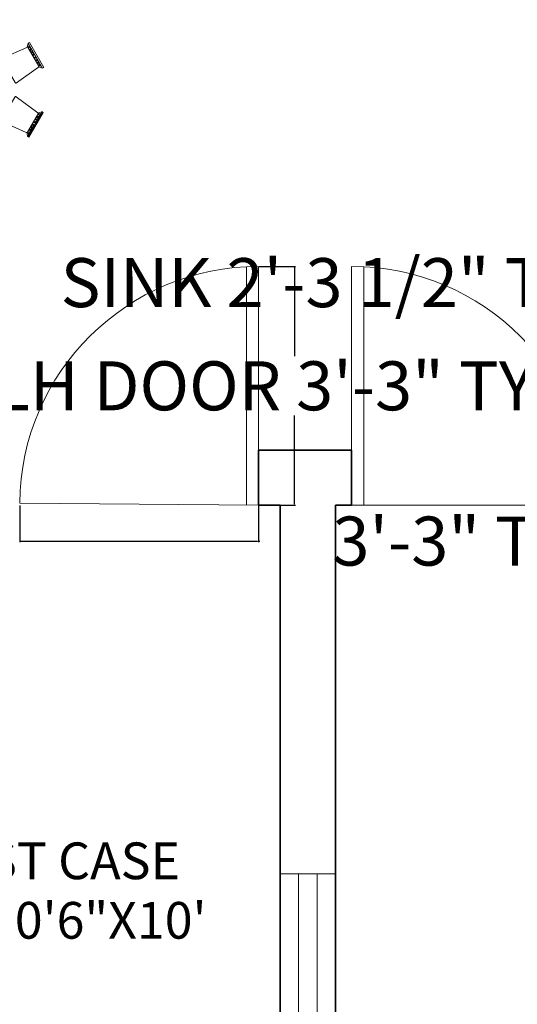
# Model space of a CAD drawing. Units: inches. Extents: x 125 to 976, y 231 to 853.
# Tile 14 of 16: x 655 to 736, y 413 to 573. Entities that reach past the tile are written whole.
import ezdxf

# ---------------------------------------------------------------- set-up
doc = ezdxf.new("R2010")
doc.units = ezdxf.units.IN
doc.header["$MEASUREMENT"] = 0
for name, color, linetype, lineweight in [('A-ANNO-DIMS', 2, 'Continuous', 18), ('A-AREA-IDEN', 7, 'Continuous', 18), ('A-DOOR', 3, 'Continuous', 18), ('A-GLAZ', 4, 'Continuous', 18), ('A-WALL', 7, 'Continuous', 35), ('Furniture', 8, 'Continuous', 15)]:
    doc.layers.add(name, color=color, linetype=linetype, lineweight=lineweight)
doc.styles.get("Standard").update_dxf_attribs({"font": 'italic8.shx'})
doc.dimstyles.get("Standard").update_dxf_attribs({"dimtxt": 8, "dimasz": 0.18, "dimexe": 0.18, "dimexo": 0.0625, "dimgap": 0.09, "dimtad": 0, "dimtih": 1, "dimtoh": 1, "dimdec": 4, "dimzin": 0, "dimdsep": 46, "dimlunit": 3, "dimtxsty": 'Standard', "dimcen": 0.09, "dimclrt": 4, "dimadec": 0, "dimazin": 0, "dimtfac": 1, "dimtdec": 4, "dimtofl": 0, "dimtmove": 0, "dimatfit": 3, "dimfxl": 1, "dimtolj": 1, "dimtzin": 0, "dimarcsym": 0})

# ---------------------------------------------------------------- blocks, each defined once
blk = doc.blocks.new('DINING-SET-ROUND-6')
for p, q in [((8.8, 22.58), (9.2, 22.26)), ((8.83, 22.8), (8.83, 22.6)), ((13.52, 22.8), (8.83, 22.8)), ((8.83, 22.6), (13.52, 22.6)), ((9.19, 22.53), (9.57, 22.55)), ((9.54, 22.27), (9.19, 22.53)), ((9.57, 22.55), (9.56, 22.32)), ((9.67, 22.56), (9.91, 22.32)), ((9.8, 22.55), (9.89, 22.55)), ((10.04, 22.32), (9.8, 22.55)), ((9.89, 22.55), (10.01, 22.45)), ((10.15, 22.56), (10.39, 22.32)), ((10.28, 22.55), (10.37, 22.55)), ((10.52, 22.32), (10.28, 22.55)), ((10.37, 22.55), (10.49, 22.45)), ((10.63, 22.56), (10.87, 22.32)), ((10.76, 22.55), (10.86, 22.55)), ((11, 22.32), (10.76, 22.55)), ((10.86, 22.55), (10.97, 22.45)), ((11.32, 22.32), (11.56, 22.55)), ((11.47, 22.55), (11.35, 22.45)), ((11.69, 22.56), (11.45, 22.32)), ((11.56, 22.55), (11.47, 22.55)), ((11.8, 22.32), (12.04, 22.55)), ((11.95, 22.55), (11.83, 22.45)), ((12.17, 22.56), (11.93, 22.32)), ((12.04, 22.55), (11.95, 22.55)), ((12.28, 22.32), (12.52, 22.55)), ((12.43, 22.55), (12.32, 22.45)), ((12.65, 22.56), (12.41, 22.32)), ((12.52, 22.55), (12.43, 22.55)), ((12.75, 22.55), (12.77, 22.32)), ((13.13, 22.53), (12.75, 22.55)), ((12.78, 22.27), (13.13, 22.53)), ((13.52, 22.58), (13.12, 22.26)), ((13.52, 22.6), (13.52, 22.8)), ((8.82, 17.72), (9.3, 22.08)), ((9.2, 22.26), (9.54, 22.27)), ((9.46, 22.23), (12.91, 22.23)), ((9.91, 22.32), (10.04, 22.32)), ((10.01, 22.45), (10.04, 22.48)), ((10.04, 22.48), (10.05, 22.34)), ((10.39, 22.32), (10.52, 22.32)), ((10.49, 22.45), (10.52, 22.48)), ((10.52, 22.48), (10.54, 22.34)), ((10.87, 22.32), (11, 22.32)), ((10.97, 22.45), (11, 22.48)), ((11, 22.48), (11.02, 22.34)), ((11.32, 22.48), (11.31, 22.34)), ((11.35, 22.45), (11.32, 22.48)), ((11.45, 22.32), (11.32, 22.32)), ((11.8, 22.48), (11.79, 22.34)), ((11.83, 22.45), (11.8, 22.48)), ((11.93, 22.32), (11.8, 22.32)), ((12.28, 22.48), (12.27, 22.34)), ((12.32, 22.45), (12.28, 22.48)), ((12.41, 22.32), (12.28, 22.32)), ((13.12, 22.26), (12.78, 22.27)), ((13.07, 22.08), (13.49, 17.72)), ((2.44, 19.22), (0.09, 15.16)), ((0.27, 15.05), (2.62, 19.11)), ((0.91, 15.41), (2.63, 18.4)), ((1.92, 17.81), (1.87, 17.73)), ((1.87, 17.73), (1.9, 17.58)), ((1.99, 17.49), (1.92, 17.81)), ((1.97, 17.93), (2.06, 17.6)), ((2.14, 18), (2.1, 17.99)), ((2.1, 17.99), (2.21, 17.9)), ((2.16, 18.23), (2.11, 18.14)), ((2.11, 18.14), (2.14, 18)), ((2.24, 17.91), (2.16, 18.23)), ((2.21, 18.35), (2.3, 18.02)), ((2.3, 18.02), (2.24, 17.91)), ((2.48, 18.75), (2.27, 18.42)), ((2.27, 18.42), (2.48, 18.32)), ((2.62, 19.11), (2.44, 19.22)), ((2.53, 18.31), (2.48, 18.75)), ((2.71, 18.6), (2.53, 18.31)), ((2.63, 19.1), (2.71, 18.6)), ((2.84, 18.46), (6.82, 16.65)), ((15.42, 16.53), (19.43, 18.29)), ((19.62, 18.97), (19.54, 18.47)), ((19.54, 18.47), (19.72, 18.18)), ((19.64, 18.23), (21.36, 15.24)), ((19.83, 19.06), (19.65, 18.95)), ((19.65, 18.95), (21.99, 14.9)), ((19.72, 18.18), (19.77, 18.62)), ((19.77, 18.62), (19.97, 18.29)), ((19.97, 18.29), (19.77, 18.19)), ((22.17, 15), (19.83, 19.06)), ((20.03, 18.21), (19.95, 17.89)), ((19.95, 17.89), (20.01, 17.77)), ((20.01, 17.77), (20.08, 18.1)), ((20.15, 17.86), (20.03, 17.77)), ((20.08, 18.1), (20.13, 18.01)), ((20.13, 18.01), (20.11, 17.87)), ((20.11, 17.87), (20.15, 17.86)), ((20.28, 17.8), (20.19, 17.47)), ((0.96, 16.18), (1.29, 16.27)), ((1.35, 16.38), (1.04, 16.28)), ((1.04, 16.28), (1.09, 16.36)), ((1.09, 16.36), (1.23, 16.41)), ((1.2, 16.59), (1.53, 16.68)), ((1.23, 16.41), (1.21, 16.46)), ((1.21, 16.46), (1.35, 16.4)), ((1.59, 16.79), (1.28, 16.7)), ((1.28, 16.7), (1.33, 16.78)), ((1.29, 16.27), (1.35, 16.38)), ((1.33, 16.78), (1.47, 16.83)), ((1.45, 16.87), (1.59, 16.82)), ((1.47, 16.83), (1.45, 16.87)), ((1.53, 16.68), (1.59, 16.79)), ((1.66, 17.16), (1.62, 17.15)), ((1.62, 17.15), (1.73, 17.07)), ((1.68, 17.39), (1.63, 17.31)), ((1.63, 17.31), (1.66, 17.16)), ((1.75, 17.07), (1.68, 17.39)), ((1.73, 17.51), (1.82, 17.18)), ((1.82, 17.18), (1.75, 17.07)), ((1.9, 17.58), (1.86, 17.57)), ((1.86, 17.57), (1.97, 17.48)), ((2.06, 17.6), (1.99, 17.49)), ((6.9, 16.42), (4.72, 12.66)), ((13.33, 17.54), (8.98, 17.54)), ((10.97, 16.52, 0.91), (10.97, 14.61, 0.91)), ((11.03, 16.52, 0.91), (10.97, 16.52, 0.91)), ((11.03, 14.61, 0.91), (11.03, 16.52, 0.91)), ((11.08, 16.52, 0.91), (11.08, 14.61, 0.91)), ((11.14, 16.52, 0.91), (11.08, 16.52, 0.91)), ((11.14, 14.61, 0.91), (11.14, 16.52, 0.91)), ((17.52, 12.54), (15.34, 16.3)), ((20.19, 17.47), (20.25, 17.36)), ((20.25, 17.36), (20.33, 17.68)), ((20.39, 17.44), (20.27, 17.35)), ((20.33, 17.68), (20.37, 17.6)), ((20.37, 17.6), (20.35, 17.45)), ((20.35, 17.45), (20.39, 17.44)), ((20.52, 17.38), (20.43, 17.05)), ((20.43, 17.05), (20.49, 16.94)), ((20.49, 16.94), (20.57, 17.26)), ((20.63, 17.02), (20.51, 16.94)), ((20.57, 17.26), (20.61, 17.18)), ((20.61, 17.18), (20.59, 17.03)), ((20.59, 17.03), (20.63, 17.02)), ((20.65, 16.66), (20.97, 16.57)), ((20.72, 16.55), (20.65, 16.66)), ((20.79, 16.74), (20.66, 16.69)), ((21.05, 16.46), (20.72, 16.55)), ((20.78, 16.7), (20.79, 16.74)), ((20.92, 16.65), (20.78, 16.7)), ((20.89, 16.25), (21.21, 16.15)), ((20.96, 16.14), (20.89, 16.25)), ((21.03, 16.33), (20.9, 16.27)), ((20.97, 16.57), (20.92, 16.65)), ((21.29, 16.05), (20.96, 16.14)), ((21.02, 16.28), (21.03, 16.33)), ((21.16, 16.23), (21.02, 16.28)), ((21.21, 16.15), (21.16, 16.23)), ((0.09, 15.16), (0.27, 15.05)), ((0.27, 15.02), (0.75, 15.21)), ((0.51, 15.33), (0.69, 15.67)), ((0.91, 15.51), (0.51, 15.33)), ((0.69, 15.67), (0.87, 15.54)), ((0.72, 15.76), (1.05, 15.85)), ((0.75, 15.21), (0.91, 15.51)), ((1.11, 15.96), (0.8, 15.86)), ((0.8, 15.86), (0.85, 15.95)), ((0.85, 15.95), (0.99, 16)), ((4.49, 12.61), (0.95, 15.2)), ((0.97, 16.04), (1.11, 15.98)), ((0.99, 16), (0.97, 16.04)), ((1.05, 15.85), (1.11, 15.96)), ((10.81, 14.88, 0.91), (10.81, 14.72, 0.91)), ((10.97, 14.88, 0.91), (10.81, 14.88, 0.91)), ((10.81, 14.72, 0.91), (10.97, 14.72, 0.91)), ((10.97, 14.61, 0.91), (11.03, 14.61, 0.91)), ((11.08, 14.88, 0.91), (11.03, 14.88, 0.91)), ((11.03, 14.72, 0.91), (11.08, 14.72, 0.91)), ((11.08, 14.61, 0.91), (11.14, 14.61, 0.91)), ((11.31, 14.88, 0.91), (11.14, 14.88, 0.91)), ((11.14, 14.72, 0.91), (11.31, 14.72, 0.91)), ((11.31, 14.72, 0.91), (11.31, 14.88, 0.91)), ((21.32, 15.03), (17.75, 12.49)), ((21.13, 15.83), (21.45, 15.73)), ((21.2, 15.72), (21.13, 15.83)), ((21.27, 15.91), (21.14, 15.85)), ((21.53, 15.63), (21.2, 15.72)), ((21.26, 15.87), (21.27, 15.91)), ((21.4, 15.82), (21.26, 15.87)), ((21.34, 15.37), (21.74, 15.2)), ((21.5, 15.07), (21.34, 15.37)), ((21.56, 15.54), (21.37, 15.41)), ((21.45, 15.73), (21.4, 15.82)), ((21.97, 14.89), (21.5, 15.07)), ((21.74, 15.2), (21.56, 15.54)), ((21.99, 14.9), (22.17, 15)), ((6.8, 13.9, 0.91), (6.77, 13.85, 0.91)), ((6.77, 13.85, 0.91), (8.43, 12.89, 0.91)), ((8.46, 12.94, 0.91), (6.8, 13.9, 0.91)), ((6.86, 14, 0.91), (6.83, 13.95, 0.91)), ((6.83, 13.95, 0.91), (8.49, 12.99, 0.91)), ((8.52, 13.04, 0.91), (6.86, 14, 0.91)), ((8.2, 13.02, 0.91), (8.12, 12.89, 0.91)), ((8.12, 12.89, 0.91), (8.26, 12.81, 0.91)), ((8.26, 13.12, 0.91), (8.23, 13.07, 0.91)), ((8.26, 12.81, 0.91), (8.34, 12.95, 0.91)), ((8.37, 13.32, 0.91), (8.29, 13.17, 0.91)), ((8.51, 13.24, 0.91), (8.37, 13.32, 0.91)), ((8.37, 13, 0.91), (8.39, 13.04, 0.91)), ((8.42, 13.1, 0.91), (8.51, 13.24, 0.91)), ((8.43, 12.89, 0.91), (8.46, 12.94, 0.91)), ((8.49, 12.99, 0.91), (8.52, 13.04, 0.91)), ((8.96, 13.32, 0.91), (8.81, 12.7, 0.91)), ((8.81, 12.7, 0.91), (9.41, 13.15, 0.91)), ((9.27, 13.54, 0.91), (8.96, 13.32, 0.91)), ((9.74, 14.31, 0.91), (9.23, 13.78, 0.91)), ((9.23, 13.78, 0.91), (9.27, 13.54, 0.91)), ((9.41, 13.15, 0.91), (9.58, 13.56, 0.91)), ((9.58, 13.56, 0.91), (9.74, 14.31, 0.91)), ((11.61, 14.37, 0.91), (10.99, 14.19, 0.91)), ((10.99, 14.19, 0.91), (11.68, 13.89, 0.91)), ((11.94, 14.21, 0.91), (11.61, 14.37, 0.91)), ((11.68, 13.89, 0.91), (12.12, 13.95, 0.91)), ((12.14, 14.36, 0.91), (11.94, 14.21, 0.91)), ((12.12, 13.95, 0.91), (12.85, 14.19, 0.91)), ((12.85, 14.19, 0.91), (12.14, 14.36, 0.91)), ((13.84, 12.59, 0.91), (13.37, 13.04, 0.91)), ((13.37, 13.04, 0.91), (13.46, 12.29, 0.91)), ((15.38, 14.23, 0.91), (13.72, 13.27, 0.91)), ((13.72, 13.27, 0.91), (13.75, 13.22, 0.91)), ((13.88, 13.54, 0.91), (13.74, 13.46, 0.91)), ((13.74, 13.46, 0.91), (13.82, 13.33, 0.91)), ((13.75, 13.22, 0.91), (15.41, 14.18, 0.91)), ((15.44, 14.13, 0.91), (13.78, 13.17, 0.91)), ((13.78, 13.17, 0.91), (13.81, 13.12, 0.91)), ((13.81, 13.12, 0.91), (15.47, 14.08, 0.91)), ((13.85, 13.27, 0.91), (13.88, 13.23, 0.91)), ((13.96, 13.4, 0.91), (13.88, 13.54, 0.91)), ((13.91, 13.18, 0.91), (13.99, 13.03, 0.91)), ((14.01, 13.31, 0.91), (13.99, 13.35, 0.91)), ((13.99, 13.03, 0.91), (14.13, 13.11, 0.91)), ((14.13, 13.11, 0.91), (14.04, 13.25, 0.91)), ((15.41, 14.18, 0.91), (15.38, 14.23, 0.91)), ((15.47, 14.08, 0.91), (15.44, 14.13, 0.91)), ((8.08, 11.67, 0.91), (8.28, 10.97, 0.91)), ((8.64, 11.17, 0.91), (8.08, 11.67, 0.91)), ((13.46, 12.29, 0.91), (13.73, 11.94, 0.91)), ((13.73, 11.94, 0.91), (14.3, 11.43, 0.91)), ((13.87, 12.23, 0.91), (13.84, 12.59, 0.91)), ((14.09, 12.13, 0.91), (13.87, 12.23, 0.91)), ((14.3, 11.43, 0.91), (14.09, 12.13, 0.91)), ((0.85, 7.79), (4.42, 10.34)), ((4.65, 10.29), (6.83, 6.52)), ((8.57, 9.99, 0.91), (6.91, 9.03, 0.91)), ((6.94, 8.97, 0.91), (8.6, 9.93, 0.91)), ((8.62, 9.89, 0.91), (6.96, 8.93, 0.91)), ((6.99, 8.88, 0.91), (8.65, 9.84, 0.91)), ((8.38, 10.07, 0.91), (8.25, 10, 0.91)), ((8.25, 10, 0.91), (8.33, 9.85, 0.91)), ((8.28, 10.97, 0.91), (8.51, 10.88, 0.91)), ((8.36, 9.8, 0.91), (8.39, 9.75, 0.91)), ((8.47, 9.93, 0.91), (8.38, 10.07, 0.91)), ((8.42, 9.7, 0.91), (8.5, 9.57, 0.91)), ((8.53, 9.83, 0.91), (8.5, 9.88, 0.91)), ((8.51, 10.88, 0.91), (8.54, 10.51, 0.91)), ((8.54, 10.51, 0.91), (9, 10.06, 0.91)), ((8.63, 9.64, 0.91), (8.56, 9.78, 0.91)), ((8.6, 9.93, 0.91), (8.57, 9.99, 0.91)), ((8.65, 9.84, 0.91), (8.62, 9.89, 0.91)), ((8.92, 10.81, 0.91), (8.64, 11.17, 0.91)), ((9, 10.06, 0.91), (8.92, 10.81, 0.91)), ((12.96, 9.95, 0.91), (12.79, 9.54, 0.91)), ((13.57, 10.41, 0.91), (12.96, 9.95, 0.91)), ((13.11, 9.57, 0.91), (13.41, 9.78, 0.91)), ((13.41, 9.78, 0.91), (13.57, 10.41, 0.91)), ((13.88, 10.12, 0.91), (13.85, 10.07, 0.91)), ((13.85, 10.07, 0.91), (15.52, 9.11, 0.91)), ((13.95, 10.01, 0.91), (13.87, 9.86, 0.91)), ((13.87, 9.86, 0.91), (14, 9.79, 0.91)), ((15.55, 9.16, 0.91), (13.88, 10.12, 0.91)), ((13.94, 10.22, 0.91), (13.91, 10.17, 0.91)), ((13.91, 10.17, 0.91), (15.57, 9.21, 0.91)), ((15.6, 9.26, 0.91), (13.94, 10.22, 0.91)), ((14.01, 10.11, 0.91), (13.98, 10.06, 0.91)), ((14, 9.79, 0.91), (14.09, 9.93, 0.91)), ((14.12, 10.3, 0.91), (14.04, 10.16, 0.91)), ((14.25, 10.22, 0.91), (14.12, 10.3, 0.91)), ((14.12, 9.98, 0.91), (14.15, 10.03, 0.91)), ((14.18, 10.08, 0.91), (14.25, 10.22, 0.91)), ((15.28, 6.4), (17.45, 10.17)), ((17.68, 10.22), (21.22, 7.62)), ((6.91, 9.03, 0.91), (6.94, 8.97, 0.91)), ((6.96, 8.93, 0.91), (6.99, 8.88, 0.91)), ((8.5, 9.57, 0.91), (8.63, 9.64, 0.91)), ((10.25, 9.16, 0.91), (9.53, 8.92, 0.91)), ((9.53, 8.92, 0.91), (10.24, 8.75, 0.91)), ((10.24, 8.75, 0.91), (10.43, 8.9, 0.91)), ((10.69, 9.22, 0.91), (10.25, 9.16, 0.91)), ((10.43, 8.9, 0.91), (10.77, 8.74, 0.91)), ((11.39, 8.92, 0.91), (10.69, 9.22, 0.91)), ((10.77, 8.74, 0.91), (11.39, 8.92, 0.91)), ((11.23, 8.39, 0.91), (11.07, 8.39, 0.91)), ((11.07, 8.39, 0.91), (11.07, 8.23, 0.91)), ((11.07, 8.23, 0.91), (11.23, 8.23, 0.91)), ((11.29, 8.5, 0.91), (11.23, 8.5, 0.91)), ((11.23, 8.5, 0.91), (11.23, 6.58, 0.91)), ((11.29, 6.58, 0.91), (11.29, 8.5, 0.91)), ((11.35, 8.39, 0.91), (11.29, 8.39, 0.91)), ((11.29, 8.23, 0.91), (11.35, 8.23, 0.91)), ((11.41, 8.5, 0.91), (11.35, 8.5, 0.91)), ((11.35, 8.5, 0.91), (11.35, 6.58, 0.91)), ((11.41, 6.58, 0.91), (11.41, 8.5, 0.91)), ((11.56, 8.39, 0.91), (11.41, 8.39, 0.91)), ((11.41, 8.23, 0.91), (11.56, 8.23, 0.91)), ((11.56, 8.23, 0.91), (11.56, 8.39, 0.91)), ((12.79, 9.54, 0.91), (12.64, 8.8, 0.91)), ((12.64, 8.8, 0.91), (13.14, 9.33, 0.91)), ((13.14, 9.33, 0.91), (13.11, 9.57, 0.91)), ((15.52, 9.11, 0.91), (15.55, 9.16, 0.91)), ((15.57, 9.21, 0.91), (15.6, 9.26, 0.91)), ((0.18, 7.93), (0, 7.82)), ((0, 7.82), (2.35, 3.77)), ((2.53, 3.87), (0.18, 7.93)), ((0.2, 7.94), (0.68, 7.75)), ((0.43, 7.63), (0.61, 7.29)), ((0.83, 7.45), (0.43, 7.63)), ((0.61, 7.29), (0.8, 7.41)), ((0.64, 7.19), (0.97, 7.11)), ((0.68, 7.75), (0.83, 7.45)), ((0.72, 7.09), (0.77, 7.01)), ((1.04, 6.99), (0.72, 7.09)), ((0.77, 7.01), (0.91, 6.96)), ((2.53, 4.6), (0.81, 7.58)), ((0.88, 6.78), (1.21, 6.69)), ((0.9, 6.91), (1.03, 6.97)), ((0.91, 6.96), (0.9, 6.91)), ((0.96, 6.67), (1.01, 6.59)), ((1.28, 6.58), (0.96, 6.67)), ((0.97, 7.11), (1.04, 6.99)), ((1.01, 6.59), (1.15, 6.54)), ((1.14, 6.5), (1.27, 6.56)), ((1.15, 6.54), (1.14, 6.5)), ((1.21, 6.69), (1.28, 6.58)), ((11.23, 6.58, 0.91), (11.29, 6.58, 0.91)), ((11.35, 6.58, 0.91), (11.41, 6.58, 0.91)), ((21.26, 7.41), (19.54, 4.43)), ((21.9, 7.77), (19.55, 3.71)), ((19.73, 3.61), (22.08, 7.67)), ((20.88, 6.56), (20.82, 6.45)), ((20.82, 6.45), (21.13, 6.54)), ((21.21, 6.65), (20.88, 6.56)), ((21.08, 6.46), (20.94, 6.41)), ((21.12, 6.98), (21.06, 6.86)), ((21.06, 6.86), (21.37, 6.96)), ((21.2, 6.78), (21.06, 6.84)), ((21.13, 6.54), (21.08, 6.46)), ((21.45, 7.06), (21.12, 6.98)), ((21.33, 6.88), (21.19, 6.83)), ((21.19, 6.83), (21.2, 6.78)), ((21.42, 7.62), (21.27, 7.32)), ((21.27, 7.32), (21.66, 7.5)), ((21.49, 7.15), (21.3, 7.28)), ((21.37, 6.96), (21.33, 6.88)), ((21.9, 7.81), (21.42, 7.62)), ((21.66, 7.5), (21.49, 7.15)), ((22.08, 7.67), (21.9, 7.77)), ((1.13, 6.36), (1.45, 6.27)), ((1.2, 6.26), (1.25, 6.17)), ((1.52, 6.16), (1.2, 6.26)), ((1.25, 6.17), (1.39, 6.12)), ((1.38, 6.08), (1.51, 6.14)), ((1.39, 6.12), (1.38, 6.08)), ((1.45, 6.27), (1.52, 6.16)), ((1.54, 5.8), (1.66, 5.89)), ((1.58, 5.79), (1.54, 5.8)), ((1.56, 5.65), (1.58, 5.79)), ((1.6, 5.56), (1.56, 5.65)), ((1.68, 5.88), (1.6, 5.56)), ((1.65, 5.44), (1.74, 5.77)), ((1.74, 5.77), (1.68, 5.88)), ((1.78, 5.39), (1.9, 5.47)), ((1.82, 5.37), (1.78, 5.39)), ((1.8, 5.23), (1.82, 5.37)), ((1.85, 5.15), (1.8, 5.23)), ((1.92, 5.47), (1.85, 5.15)), ((1.9, 5.03), (1.98, 5.35)), ((1.98, 5.35), (1.92, 5.47)), ((2.02, 4.97), (2.14, 5.06)), ((2.07, 4.96), (2.02, 4.97)), ((2.04, 4.81), (2.07, 4.96)), ((2.16, 5.05), (2.09, 4.73)), ((2.14, 4.61), (2.22, 4.94)), ((2.22, 4.94), (2.16, 5.05)), ((6.75, 6.3), (2.74, 4.53)), ((9.1, 0.74), (8.68, 5.1)), ((9.14, 0.73), (8.73, 5.09)), ((8.84, 5.28), (13.19, 5.28)), ((8.89, 5.26), (13.23, 5.26)), ((13.35, 5.1), (12.87, 0.74)), ((13.39, 5.09), (12.91, 0.72)), ((19.33, 4.36), (15.35, 6.18)), ((19.87, 4.81), (19.94, 4.92)), ((19.94, 4.92), (20.01, 4.6)), ((20.07, 4.84), (19.96, 4.92)), ((20.03, 4.83), (20.07, 4.84)), ((20.06, 4.68), (20.03, 4.83)), ((20.11, 5.22), (20.18, 5.34)), ((20.2, 4.9), (20.11, 5.22)), ((20.18, 5.34), (20.25, 5.01)), ((20.31, 5.26), (20.2, 5.34)), ((20.25, 5.01), (20.3, 5.1)), ((20.27, 5.24), (20.31, 5.26)), ((20.3, 5.1), (20.27, 5.24)), ((20.35, 5.64), (20.42, 5.75)), ((20.44, 5.31), (20.35, 5.64)), ((20.42, 5.75), (20.49, 5.43)), ((20.56, 5.67), (20.44, 5.76)), ((20.49, 5.43), (20.54, 5.51)), ((20.51, 5.66), (20.56, 5.67)), ((20.54, 5.51), (20.51, 5.66)), ((20.64, 6.14), (20.58, 6.03)), ((20.58, 6.03), (20.89, 6.13)), ((20.72, 5.95), (20.58, 6.01)), ((20.97, 6.23), (20.64, 6.14)), ((20.84, 6.04), (20.7, 5.99)), ((20.7, 5.99), (20.72, 5.95)), ((20.96, 6.37), (20.82, 6.43)), ((20.89, 6.13), (20.84, 6.04)), ((20.94, 6.41), (20.96, 6.37)), ((2.09, 4.73), (2.04, 4.81)), ((2.2, 4.53), (2.4, 4.63)), ((2.4, 4.21), (2.2, 4.53)), ((2.35, 3.77), (2.53, 3.87)), ((2.45, 4.64), (2.4, 4.21)), ((2.63, 4.36), (2.45, 4.64)), ((2.56, 3.85), (2.63, 4.36)), ((19.46, 4.23), (19.64, 4.51)), ((19.54, 3.72), (19.46, 4.23)), ((19.55, 3.71), (19.73, 3.61)), ((19.64, 4.51), (19.69, 4.08)), ((19.9, 4.4), (19.69, 4.5)), ((19.69, 4.08), (19.9, 4.4)), ((19.96, 4.48), (19.87, 4.81)), ((20.01, 4.6), (20.06, 4.68)), ((8.65, 0.24), (9.05, 0.57)), ((8.65, 0.23), (8.65, 0.02)), ((13.34, 0.23), (8.65, 0.23)), ((8.65, 0.02), (13.34, 0.02)), ((8.69, 0.23), (9.09, 0.55)), ((8.69, 0.21), (8.69, 0)), ((13.38, 0.21), (8.69, 0.21)), ((8.69, 0), (13.38, 0)), ((9.39, 0.55), (9.04, 0.29)), ((9.04, 0.29), (9.42, 0.28)), ((9.05, 0.57), (9.39, 0.55)), ((9.43, 0.53), (9.08, 0.28)), ((9.08, 0.28), (9.46, 0.26)), ((9.09, 0.55), (9.43, 0.53)), ((12.71, 0.6), (9.26, 0.6)), ((12.75, 0.58), (9.3, 0.58)), ((9.42, 0.28), (9.41, 0.5)), ((9.46, 0.26), (9.45, 0.49)), ((9.52, 0.26), (9.76, 0.5)), ((9.56, 0.25), (9.8, 0.49)), ((9.89, 0.5), (9.65, 0.28)), ((9.65, 0.28), (9.74, 0.28)), ((9.93, 0.49), (9.69, 0.26)), ((9.69, 0.26), (9.78, 0.26)), ((9.74, 0.28), (9.85, 0.37)), ((9.76, 0.5), (9.89, 0.5)), ((9.78, 0.26), (9.9, 0.36)), ((9.8, 0.49), (9.93, 0.49)), ((9.85, 0.37), (9.89, 0.34)), ((9.89, 0.34), (9.9, 0.49)), ((9.9, 0.36), (9.93, 0.33)), ((9.93, 0.33), (9.94, 0.47)), ((10, 0.26), (10.24, 0.5)), ((10.04, 0.25), (10.28, 0.49)), ((10.37, 0.5), (10.13, 0.28)), ((10.13, 0.28), (10.22, 0.28)), ((10.41, 0.49), (10.17, 0.26)), ((10.17, 0.26), (10.27, 0.26)), ((10.22, 0.28), (10.34, 0.37)), ((10.24, 0.5), (10.37, 0.5)), ((10.27, 0.26), (10.38, 0.36)), ((10.28, 0.49), (10.41, 0.49)), ((10.34, 0.37), (10.37, 0.34)), ((10.37, 0.34), (10.38, 0.49)), ((10.38, 0.36), (10.41, 0.33)), ((10.41, 0.33), (10.43, 0.47)), ((10.48, 0.26), (10.72, 0.5)), ((10.52, 0.25), (10.76, 0.49)), ((10.85, 0.5), (10.61, 0.28)), ((10.61, 0.28), (10.71, 0.28)), ((10.89, 0.49), (10.65, 0.26)), ((10.65, 0.26), (10.75, 0.26)), ((10.71, 0.28), (10.82, 0.37)), ((10.72, 0.5), (10.85, 0.5)), ((10.75, 0.26), (10.86, 0.36)), ((10.76, 0.49), (10.89, 0.49)), ((10.82, 0.37), (10.85, 0.34)), ((10.85, 0.34), (10.87, 0.49)), ((10.86, 0.36), (10.89, 0.33)), ((10.89, 0.33), (10.91, 0.47)), ((11.17, 0.34), (11.15, 0.49)), ((11.17, 0.5), (11.41, 0.28)), ((11.3, 0.5), (11.17, 0.5)), ((11.2, 0.37), (11.17, 0.34)), ((11.21, 0.33), (11.2, 0.47)), ((11.31, 0.28), (11.2, 0.37)), ((11.21, 0.49), (11.45, 0.26)), ((11.34, 0.49), (11.21, 0.49)), ((11.24, 0.36), (11.21, 0.33)), ((11.36, 0.26), (11.24, 0.36)), ((11.54, 0.26), (11.3, 0.5)), ((11.41, 0.28), (11.31, 0.28)), ((11.58, 0.25), (11.34, 0.49)), ((11.45, 0.26), (11.36, 0.26)), ((11.65, 0.34), (11.64, 0.49)), ((11.65, 0.5), (11.89, 0.28)), ((11.78, 0.5), (11.65, 0.5)), ((11.68, 0.37), (11.65, 0.34)), ((11.69, 0.33), (11.68, 0.47)), ((11.8, 0.28), (11.68, 0.37)), ((11.69, 0.49), (11.93, 0.26)), ((11.82, 0.49), (11.69, 0.49)), ((11.73, 0.36), (11.69, 0.33)), ((11.84, 0.26), (11.73, 0.36)), ((12.02, 0.26), (11.78, 0.5)), ((11.89, 0.28), (11.8, 0.28)), ((12.06, 0.25), (11.82, 0.49)), ((11.93, 0.26), (11.84, 0.26)), ((12.13, 0.34), (12.12, 0.49)), ((12.13, 0.5), (12.37, 0.28)), ((12.26, 0.5), (12.13, 0.5)), ((12.17, 0.37), (12.13, 0.34)), ((12.17, 0.33), (12.16, 0.47)), ((12.17, 0.49), (12.42, 0.26)), ((12.3, 0.49), (12.17, 0.49)), ((12.28, 0.28), (12.17, 0.37)), ((12.21, 0.36), (12.17, 0.33)), ((12.32, 0.26), (12.21, 0.36)), ((12.5, 0.26), (12.26, 0.5)), ((12.37, 0.28), (12.28, 0.28)), ((12.54, 0.25), (12.3, 0.49)), ((12.42, 0.26), (12.32, 0.26)), ((12.6, 0.28), (12.61, 0.5)), ((12.98, 0.29), (12.6, 0.28)), ((12.97, 0.57), (12.63, 0.55)), ((12.63, 0.55), (12.98, 0.29)), ((12.64, 0.26), (12.66, 0.49)), ((13.02, 0.28), (12.64, 0.26)), ((13.01, 0.55), (12.67, 0.53)), ((12.67, 0.53), (13.02, 0.28)), ((13.37, 0.24), (12.97, 0.57)), ((13.41, 0.23), (13.01, 0.55)), ((13.34, 0.02), (13.34, 0.23)), ((13.38, 0), (13.38, 0.21))]:
    blk.add_line(p, q)
for centre, radius in [((11.09, 11.41), 5.4), ((11.09, 11.41), 5.3), ((8.3, 14.2, 0.91), 0.616), ((10.11, 15.33, 0.91), 0.572), ((10.13, 15.34, 0.91), 0.295), ((12.04, 15.38, 0.91), 0.616), ((13.92, 14.37, 0.91), 0.572), ((13.94, 14.37, 0.91), 0.295), ((7.38, 12.51, 0.91), 0.572), ((14.93, 12.73, 0.91), 0.616), ((7.38, 12.53, 0.91), 0.295), ((7.45, 10.38, 0.91), 0.616), ((15, 10.59, 0.91), 0.572), ((15, 10.58, 0.91), 0.295), ((8.45, 8.73, 0.91), 0.572), ((8.44, 8.74, 0.91), 0.295), ((10.34, 7.73, 0.91), 0.616), ((12.26, 7.77, 0.91), 0.572), ((12.25, 7.77, 0.91), 0.295), ((14.08, 8.9, 0.91), 0.616)]:
    blk.add_circle(centre, radius)
for centre, radius, start, end in [((9.46, 22.07), 0.16, 90, 173.7428), ((12.91, 22.07), 0.16, 5.4801, 90), ((2.77, 18.32), 0.16, 65.4801, 150), ((8.98, 17.7), 0.16, 173.7428, 270), ((13.33, 17.7), 0.16, 270, 5.4801), ((19.5, 18.15), 0.16, 30, 113.7428), ((6.76, 16.5), 0.16, 330, 65.4801), ((15.48, 16.38), 0.16, 113.7428, 210), ((1.05, 15.33), 0.16, 150, 233.7428), ((11.86, 14.13, 0.91), 0.448, 26.6641, 154.1442), ((21.22, 15.16), 0.16, 305.4801, 30), ((9.3, 13.42, 0.91), 0.448, 86.6641, 214.1442), ((9.3, 13.42, 0.91), 0.448, 257.0611, 44.0662), ((11.86, 14.13, 0.91), 0.448, 197.0611, 344.0662), ((4.58, 12.74), 0.16, 233.7428, 330), ((8.62, 10.85, 0.91), 0.448, 317.0611, 104.0662), ((13.76, 12.26, 0.91), 0.448, 137.0611, 284.0662), ((13.76, 12.26, 0.91), 0.448, 326.6641, 94.1442), ((17.66, 12.62), 0.16, 210, 305.4801), ((4.52, 10.21), 0.16, 30, 125.4801), ((8.62, 10.85, 0.91), 0.448, 146.6641, 274.1442), ((13.08, 9.68, 0.91), 0.448, 77.0611, 224.0662), ((13.08, 9.68, 0.91), 0.448, 266.6641, 34.1442), ((17.59, 10.09), 0.16, 53.7428, 150), ((10.51, 8.98, 0.91), 0.448, 17.0611, 164.0662), ((10.51, 8.98, 0.91), 0.448, 206.6641, 334.1442), ((0.95, 7.66), 0.16, 125.4801, 210), ((6.69, 6.44), 0.16, 293.7428, 30), ((21.13, 7.49), 0.16, 330, 53.7428), ((8.84, 5.12), 0.16, 90, 185.4801), ((8.89, 5.1), 0.16, 90, 185.4801), ((13.19, 5.12), 0.16, 353.7428, 90), ((13.23, 5.1), 0.16, 353.7428, 90), ((15.41, 6.32), 0.16, 150, 245.4801), ((2.67, 4.68), 0.16, 210, 293.7428), ((19.4, 4.51), 0.16, 245.4801, 330), ((9.26, 0.76), 0.16, 185.4801, 270), ((9.3, 0.74), 0.16, 185.4801, 270), ((12.71, 0.76), 0.16, 270, 353.7428), ((12.75, 0.74), 0.16, 270, 353.7428)]:
    blk.add_arc(centre, radius, start, end)
blk = doc.blocks.new('WINDOW-48IN')
for p, q in [((0, 0), (0, 48)), ((0, 48), (9, 48)), ((3, 0), (3, 48)), ((6, 0), (6, 48)), ((9, 48), (9, 0)), ((9, 0), (0, 0))]:
    blk.add_line(p, q)
blk = doc.blocks.new('DOOR-39IN-LH')
for p, q in [((-2, 0), (-2, 38.95)), ((0, 0), (0, 39)), ((-39, 0.34), (0, 0))]:
    blk.add_line(p, q)
blk.add_arc((0, 0), 39, 90, 179.5065)
blk = doc.blocks.new('DOOR-39IN-RH')
for p, q in [((0, 39), (0, 0)), ((2, 38.95), (2, 0)), ((0, 0), (39, 0))]:
    blk.add_line(p, q)
blk.add_arc((0, 0), 39, 0, 90)
blk = doc.blocks.new('*D38')
at = {"layer": 'A-ANNO-DIMS', "color": 0, "lineweight": -2, "transparency": 16777216}
for p, q in [((694.22, 533.1), (700.18, 533.1)), ((700, 532.92), (700, 518.46)), ((700, 494.28), (700, 508.75)), ((694.22, 494.1), (700.18, 494.1))]:
    blk.add_line(p, q, dxfattribs=at)
at = {"layer": 'A-ANNO-DIMS', "color": 0, "transparency": 16777216}
for points in [[(699.97, 532.92), (700.03, 532.92), (700, 533.1)], [(699.97, 494.28), (700.03, 494.28), (700, 494.1)]]:
    blk.add_solid(points, dxfattribs=at)
at = {"layer": 'Defpoints', "color": 0, "transparency": 16777216}
for p in [(694.15, 533.1), (700, 533.1), (694.15, 494.1)]:
    blk.add_point(p, dxfattribs=at)
at = {"layer": 'A-ANNO-DIMS', "color": 4, "transparency": 16777216, "insert": (700, 513.6), "char_height": 8, "attachment_point": 5}
blk.add_mtext('\\A1;LH DOOR 3\'-3" TYP.', dxfattribs=at)
blk = doc.blocks.new('*D39')
at = {"layer": 'A-ANNO-DIMS', "color": 0, "lineweight": -2, "transparency": 16777216}
for p, q in [((655.15, 494.04), (655.15, 488.07)), ((694.15, 494.04), (694.15, 488.07)), ((655.33, 488.25), (693.97, 488.25)), ((694.15, 488.25), (694.33, 488.25))]:
    blk.add_line(p, q, dxfattribs=at)
at = {"layer": 'A-ANNO-DIMS', "color": 0, "transparency": 16777216}
for points in [[(655.33, 488.28), (655.33, 488.22), (655.15, 488.25)], [(693.97, 488.28), (693.97, 488.22), (694.15, 488.25)]]:
    blk.add_solid(points, dxfattribs=at)
at = {"layer": 'Defpoints', "color": 0, "transparency": 16777216}
for p in [(655.15, 494.1), (694.15, 494.1), (694.15, 488.25)]:
    blk.add_point(p, dxfattribs=at)
at = {"layer": 'A-ANNO-DIMS', "color": 4, "transparency": 16777216, "insert": (730.61, 488.25), "char_height": 8, "attachment_point": 5}
blk.add_mtext('\\A1;3\'-3" TYP.', dxfattribs=at)
blk = doc.blocks.new('*D48')
at = {"layer": 'A-ANNO-DIMS', "color": 0, "lineweight": -2, "transparency": 16777216}
for p, q in [((609.57, 526.38), (609.57, 530.63)), ((637.13, 526.38), (637.13, 530.63)), ((609.75, 530.45), (636.95, 530.45)), ((637.13, 530.45), (637.31, 530.45))]:
    blk.add_line(p, q, dxfattribs=at)
at = {"layer": 'A-ANNO-DIMS', "color": 0, "transparency": 16777216}
for points in [[(609.75, 530.48), (609.75, 530.42), (609.57, 530.45)], [(636.95, 530.48), (636.95, 530.42), (637.13, 530.45)]]:
    blk.add_solid(points, dxfattribs=at)
at = {"layer": 'Defpoints', "color": 0, "transparency": 16777216}
for p in [(637.13, 530.45), (609.57, 526.32), (637.13, 526.32)]:
    blk.add_point(p, dxfattribs=at)
at = {"layer": 'A-ANNO-DIMS', "color": 4, "transparency": 16777216, "insert": (709.21, 530.45), "char_height": 8, "attachment_point": 5}
blk.add_mtext('\\A1;SINK 2\'-3 1/2" TYP.', dxfattribs=at)

msp = doc.modelspace()

# ---------------------------------------------------------------- linework, layer by layer
at = {"layer": 'A-WALL'}
for p, q in [((694.15273, 494.10475), (694.15273, 503.10475)), ((709.30979, 503.10475), (694.15273, 503.10475)), ((709.30979, 494.10475), (709.30979, 503.10475)), ((697.69287, 494.10475), (694.15273, 494.10475)), ((697.69287, 494.10475), (697.69287, 332.10475)), ((706.69287, 494.10475), (706.69287, 338.10475)), ((709.30979, 494.10475), (706.69287, 494.10475))]:
    msp.add_line(p, q, dxfattribs=at)

# ---------------------------------------------------------------- block references
at = {"layer": 'A-DOOR'}
for name, p in [('DOOR-39IN-LH', (694.15273, 494.10475)), ('DOOR-39IN-RH', (709.30979, 494.10475))]:
    msp.add_blockref(name, p, dxfattribs=at)
at = {"layer": 'A-GLAZ'}
msp.add_blockref('WINDOW-48IN', (697.69, 385.91728), dxfattribs=at)
at = {"layer": 'Furniture'}
msp.add_blockref('DINING-SET-ROUND-6', (636.90561, 550.58741), dxfattribs=at)

# ---------------------------------------------------------------- texts
at = {"layer": 'A-AREA-IDEN'}
for s, p in [('ST CASE', (649.81476, 433.03507)), ('10\'6"X10\'', (649.81476, 423.32078))]:
    msp.add_text(s, height=6, dxfattribs=at).set_placement(p)

# ---------------------------------------------------------------- dimensions: what is measured, and where the dimension line sits
at = {"layer": 'A-ANNO-DIMS'}
for base, p1, p2, text, picture, middle in [((637.12727, 530.45033), (609.56827, 526.31648), (637.12727, 526.31648), 'SINK <> TYP.', '*D48', (709.2068, 530.45033)), ((694.15273, 488.25475), (655.15418, 494.10475), (694.15273, 494.10475), '<> TYP.', '*D39', (730.61321, 488.25475))]:
    dim = msp.add_linear_dim(base=base, p1=p1, p2=p2, text=text, dimstyle='Standard', override={"dimdec": 1, "dimlfac": 1, "dimrnd": 0, "dimzin": 1, "dimdsep": 46, "dimlunit": 4, "dimfrac": 2}, dxfattribs=at)
    dim.commit()
    dim.dimension.update_dxf_attribs({"geometry": picture, "text_midpoint": middle})
dim = msp.add_linear_dim(base=(700.00273, 533.10475), p1=(694.15273, 494.10475), p2=(694.15273, 533.10475), angle=90, text='LH DOOR <> TYP.', dimstyle='Standard', override={"dimdec": 1, "dimlfac": 1, "dimrnd": 0, "dimzin": 1, "dimdsep": 46, "dimlunit": 4, "dimfrac": 2}, dxfattribs=at)
dim.commit()
dim.dimension.update_dxf_attribs({"geometry": '*D38', "text_midpoint": (700.00273, 513.60475)})

doc.saveas('drawing.dxf')
